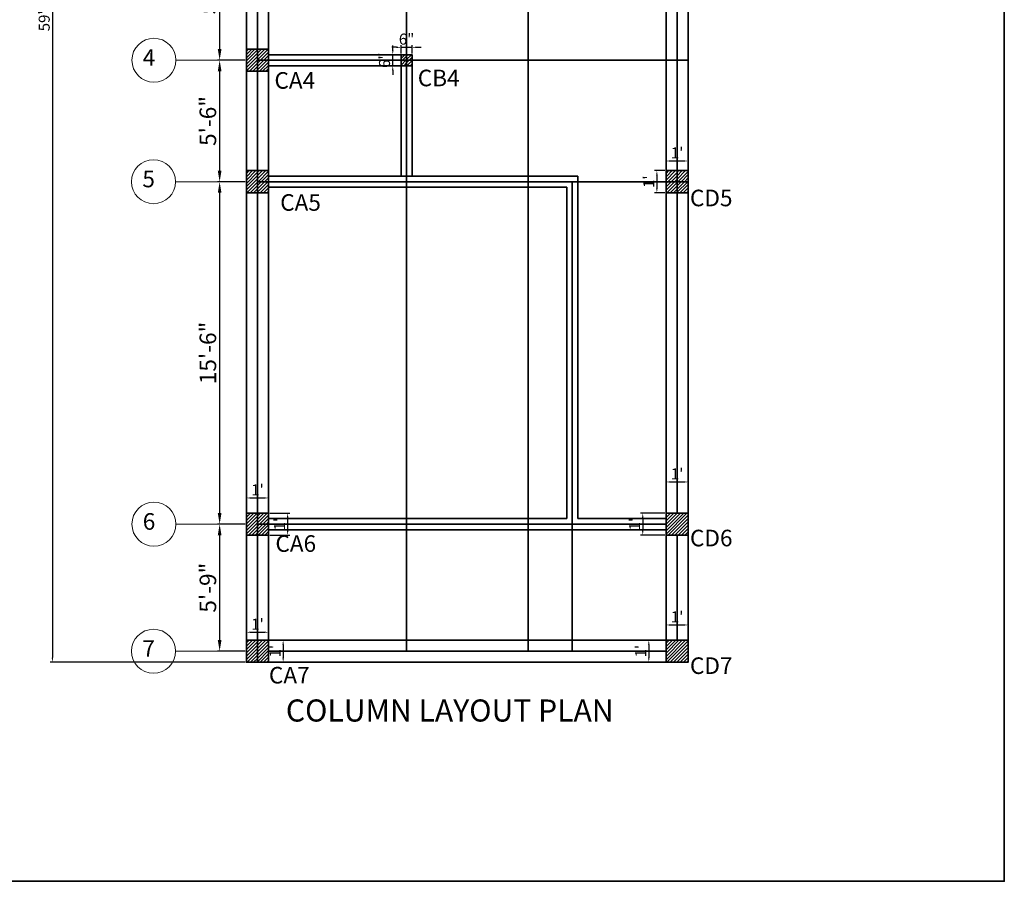
# Model space of a CAD drawing. Units: millimetres. Extents: x 20768 to 23556, y 50760 to 52704.
# Tile 34 of 36: x 23021 to 23556, y 51624 to 52092. Entities that reach past the tile are written whole.
import ezdxf

# ---------------------------------------------------------------- set-up
doc = ezdxf.new("R2010")
doc.units = ezdxf.units.MM
for name, color, linetype, lineweight in [('A-ANNO-TTLB', 7, 'Continuous', 35), ('S-ANNO-DIMS', 2, 'Continuous', 18), ('S-ANNO-TEXT', 6, 'Continuous', 18), ('S-BEAM', 3, 'Continuous', 35), ('S-COLS', 20, 'Continuous', 35), ('S-COLS-PATT', 8, 'Continuous', 13), ('S-GRID', 1, 'Continuous', 18)]:
    doc.layers.add(name, color=color, linetype=linetype, lineweight=lineweight)
doc.styles.get("Standard").update_dxf_attribs({"font": 'arial.ttf'})
doc.dimstyles.new('ISO-25', dxfattribs={"dimtxt": 6, "dimasz": 2.5, "dimexe": 1.25, "dimexo": 0.625, "dimtad": 1, "dimdec": 0, "dimlunit": 3, "dimtxsty": 'Standard', "dimcen": 2.5, "dimadec": 0, "dimazin": 0, "dimtfac": 1, "dimtdec": 0, "dimtmove": 0, "dimatfit": 3, "dimfxl": 1, "dimarcsym": 0})
pattern_1 = [(45, (1088.7427, 0), (-0.898025612, 0.898025612), [])]

# ---------------------------------------------------------------- blocks, each defined once
blk = doc.blocks.new('*D85')
at = {"layer": 'Defpoints', "color": 0, "transparency": 16777216}
for p in [(23144.01, 52129.51), (23129.44, 52069.51), (23144.01, 52069.51)]:
    blk.add_point(p, dxfattribs=at)
at = {"layer": 'S-ANNO-DIMS', "color": 0, "lineweight": -2, "transparency": 16777216}
for p, q in [((23143.39, 52129.51), (23128.19, 52129.51)), ((23129.44, 52123.51), (23129.44, 52075.51)), ((23143.39, 52069.51), (23128.19, 52069.51))]:
    blk.add_line(p, q, dxfattribs=at)
at = {"layer": 'S-ANNO-DIMS', "color": 0, "transparency": 16777216}
for points in [[(23128.44, 52123.51), (23130.44, 52123.51), (23129.44, 52129.51)], [(23128.44, 52075.51), (23130.44, 52075.51), (23129.44, 52069.51)]]:
    blk.add_solid(points, dxfattribs=at)
at = {"layer": 'S-ANNO-DIMS', "color": 0, "transparency": 16777216, "insert": (23124.24, 52099.51), "char_height": 9, "attachment_point": 5, "rotation": 90}
blk.add_mtext("5'", dxfattribs=at)
blk = doc.blocks.new('*D86')
at = {"layer": 'Defpoints', "color": 0, "transparency": 16777216}
for p in [(23144.01, 52069.51), (23129.44, 52003.51), (23144.01, 52003.51)]:
    blk.add_point(p, dxfattribs=at)
at = {"layer": 'S-ANNO-DIMS', "color": 0, "lineweight": -2, "transparency": 16777216}
for p, q in [((23143.39, 52069.51), (23128.19, 52069.51)), ((23129.44, 52063.51), (23129.44, 52009.51)), ((23143.39, 52003.51), (23128.19, 52003.51))]:
    blk.add_line(p, q, dxfattribs=at)
at = {"layer": 'S-ANNO-DIMS', "color": 0, "transparency": 16777216}
for points in [[(23128.44, 52063.51), (23130.44, 52063.51), (23129.44, 52069.51)], [(23128.44, 52009.51), (23130.44, 52009.51), (23129.44, 52003.51)]]:
    blk.add_solid(points, dxfattribs=at)
at = {"layer": 'S-ANNO-DIMS', "color": 0, "transparency": 16777216, "insert": (23124.22, 52036.51), "char_height": 9, "attachment_point": 5, "rotation": 90}
blk.add_mtext('5\'-6"', dxfattribs=at)
blk = doc.blocks.new('*D87')
at = {"layer": 'Defpoints', "color": 0, "transparency": 16777216}
for p in [(23144.01, 52003.51), (23129.44, 51817.51), (23144.01, 51817.51)]:
    blk.add_point(p, dxfattribs=at)
at = {"layer": 'S-ANNO-DIMS', "color": 0, "lineweight": -2, "transparency": 16777216}
for p, q in [((23143.39, 52003.51), (23128.19, 52003.51)), ((23129.44, 51997.51), (23129.44, 51823.51)), ((23143.39, 51817.51), (23128.19, 51817.51))]:
    blk.add_line(p, q, dxfattribs=at)
at = {"layer": 'S-ANNO-DIMS', "color": 0, "transparency": 16777216}
for points in [[(23128.44, 51997.51), (23130.44, 51997.51), (23129.44, 52003.51)], [(23128.44, 51823.51), (23130.44, 51823.51), (23129.44, 51817.51)]]:
    blk.add_solid(points, dxfattribs=at)
at = {"layer": 'S-ANNO-DIMS', "color": 0, "transparency": 16777216, "insert": (23124.22, 51910.51), "char_height": 9, "attachment_point": 5, "rotation": 90}
blk.add_mtext('15\'-6"', dxfattribs=at)
blk = doc.blocks.new('*D88')
at = {"layer": 'Defpoints', "color": 0, "transparency": 16777216}
for p in [(23144.01, 51817.51), (23129.44, 51748.51), (23144.01, 51748.51)]:
    blk.add_point(p, dxfattribs=at)
at = {"layer": 'S-ANNO-DIMS', "color": 0, "lineweight": -2, "transparency": 16777216}
for p, q in [((23143.39, 51817.51), (23128.19, 51817.51)), ((23129.44, 51811.51), (23129.44, 51754.51)), ((23143.39, 51748.51), (23128.19, 51748.51))]:
    blk.add_line(p, q, dxfattribs=at)
at = {"layer": 'S-ANNO-DIMS', "color": 0, "transparency": 16777216}
for points in [[(23128.44, 51811.51), (23130.44, 51811.51), (23129.44, 51817.51)], [(23128.44, 51754.51), (23130.44, 51754.51), (23129.44, 51748.51)]]:
    blk.add_solid(points, dxfattribs=at)
at = {"layer": 'S-ANNO-DIMS', "color": 0, "transparency": 16777216, "insert": (23124.22, 51783.01), "char_height": 9, "attachment_point": 5, "rotation": 90}
blk.add_mtext('5\'-9"', dxfattribs=at)
blk = doc.blocks.new('*D96')
at = {"layer": 'Defpoints', "color": 0, "transparency": 16777216}
for p in [(23228.01, 52072.51), (23234.01, 52076.5), (23234.01, 52072.51)]:
    blk.add_point(p, dxfattribs=at)
at = {"layer": 'S-ANNO-DIMS', "color": 0, "lineweight": -2, "transparency": 16777216}
for p, q in [((23228.01, 52073.13), (23228.01, 52077.75)), ((23234.01, 52073.13), (23234.01, 52077.75)), ((23225.51, 52076.5), (23223.01, 52076.5)), ((23228.01, 52076.5), (23234.01, 52076.5)), ((23236.51, 52076.5), (23239.01, 52076.5))]:
    blk.add_line(p, q, dxfattribs=at)
at = {"layer": 'S-ANNO-DIMS', "color": 0, "transparency": 16777216}
for points in [[(23225.51, 52076.92), (23225.51, 52076.09), (23228.01, 52076.5)], [(23236.51, 52076.92), (23236.51, 52076.09), (23234.01, 52076.5)]]:
    blk.add_solid(points, dxfattribs=at)
at = {"layer": 'S-ANNO-DIMS', "color": 0, "transparency": 16777216, "insert": (23231.01, 52080.19), "char_height": 6, "attachment_point": 5}
blk.add_mtext('6"', dxfattribs=at)
blk = doc.blocks.new('*D97')
at = {"layer": 'Defpoints', "color": 0, "transparency": 16777216}
for p in [(23223.5, 52072.51), (23228.01, 52072.51), (23228.01, 52066.51)]:
    blk.add_point(p, dxfattribs=at)
at = {"layer": 'S-ANNO-DIMS', "color": 0, "lineweight": -2, "transparency": 16777216}
for p, q in [((23227.39, 52072.51), (23222.25, 52072.51)), ((23223.5, 52075.01), (23223.5, 52077.51)), ((23223.5, 52066.51), (23223.5, 52072.51)), ((23227.39, 52066.51), (23222.25, 52066.51)), ((23223.5, 52064.01), (23223.5, 52061.51))]:
    blk.add_line(p, q, dxfattribs=at)
at = {"layer": 'S-ANNO-DIMS', "color": 0, "transparency": 16777216}
for points in [[(23223.09, 52075.01), (23223.92, 52075.01), (23223.5, 52072.51)], [(23223.09, 52064.01), (23223.92, 52064.01), (23223.5, 52066.51)]]:
    blk.add_solid(points, dxfattribs=at)
at = {"layer": 'S-ANNO-DIMS', "color": 0, "transparency": 16777216, "insert": (23219.81, 52069.51), "char_height": 6, "attachment_point": 5, "rotation": 90}
blk.add_mtext('6"', dxfattribs=at)
blk = doc.blocks.new('*D98')
at = {"layer": 'Defpoints', "color": 0, "transparency": 16777216}
for p in [(23384.01, 52014.76), (23372.01, 52009.51), (23384.01, 52009.51)]:
    blk.add_point(p, dxfattribs=at)
at = {"layer": 'S-ANNO-DIMS', "color": 0, "lineweight": -2, "transparency": 16777216}
for p, q in [((23372.01, 52010.13), (23372.01, 52016.01)), ((23374.51, 52014.76), (23381.51, 52014.76)), ((23384.01, 52010.13), (23384.01, 52016.01))]:
    blk.add_line(p, q, dxfattribs=at)
at = {"layer": 'S-ANNO-DIMS', "color": 0, "transparency": 16777216}
for points in [[(23374.51, 52015.17), (23374.51, 52014.34), (23372.01, 52014.76)], [(23381.51, 52015.17), (23381.51, 52014.34), (23384.01, 52014.76)]]:
    blk.add_solid(points, dxfattribs=at)
at = {"layer": 'S-ANNO-DIMS', "color": 0, "transparency": 16777216, "insert": (23378.01, 52018.39), "char_height": 6, "attachment_point": 5}
blk.add_mtext("1'", dxfattribs=at)
blk = doc.blocks.new('*D99')
at = {"layer": 'Defpoints', "color": 0, "transparency": 16777216}
for p in [(23372.01, 52009.51), (23367.02, 51997.51), (23372.01, 51997.51)]:
    blk.add_point(p, dxfattribs=at)
at = {"layer": 'S-ANNO-DIMS', "color": 0, "lineweight": -2, "transparency": 16777216}
for p, q in [((23371.39, 52009.51), (23365.77, 52009.51)), ((23367.02, 52007.01), (23367.02, 52000.01)), ((23371.39, 51997.51), (23365.77, 51997.51))]:
    blk.add_line(p, q, dxfattribs=at)
at = {"layer": 'S-ANNO-DIMS', "color": 0, "transparency": 16777216}
for points in [[(23366.61, 52007.01), (23367.44, 52007.01), (23367.02, 52009.51)], [(23366.61, 52000.01), (23367.44, 52000.01), (23367.02, 51997.51)]]:
    blk.add_solid(points, dxfattribs=at)
at = {"layer": 'S-ANNO-DIMS', "color": 0, "transparency": 16777216, "insert": (23363.39, 52003.51), "char_height": 6, "attachment_point": 5, "rotation": 90}
blk.add_mtext("1'", dxfattribs=at)
blk = doc.blocks.new('*D100')
at = {"layer": 'Defpoints', "color": 0, "transparency": 16777216}
for p in [(23384.01, 51762.75), (23372.01, 51754.51), (23384.01, 51754.51)]:
    blk.add_point(p, dxfattribs=at)
at = {"layer": 'S-ANNO-DIMS', "color": 0, "lineweight": -2, "transparency": 16777216}
for p, q in [((23372.01, 51755.13), (23372.01, 51764)), ((23374.51, 51762.75), (23381.51, 51762.75)), ((23384.01, 51755.13), (23384.01, 51764))]:
    blk.add_line(p, q, dxfattribs=at)
at = {"layer": 'S-ANNO-DIMS', "color": 0, "transparency": 16777216}
for points in [[(23374.51, 51763.17), (23374.51, 51762.33), (23372.01, 51762.75)], [(23381.51, 51763.17), (23381.51, 51762.33), (23384.01, 51762.75)]]:
    blk.add_solid(points, dxfattribs=at)
at = {"layer": 'S-ANNO-DIMS', "color": 0, "transparency": 16777216, "insert": (23378.01, 51766.39), "char_height": 6, "attachment_point": 5}
blk.add_mtext("1'", dxfattribs=at)
blk = doc.blocks.new('*D101')
at = {"layer": 'Defpoints', "color": 0, "transparency": 16777216}
for p in [(23372.01, 51754.51), (23362.63, 51742.51), (23372.01, 51742.51)]:
    blk.add_point(p, dxfattribs=at)
at = {"layer": 'S-ANNO-DIMS', "color": 0, "lineweight": -2, "transparency": 16777216}
for p, q in [((23371.39, 51754.51), (23361.38, 51754.51)), ((23362.63, 51752.01), (23362.63, 51745.01)), ((23371.39, 51742.51), (23361.38, 51742.51))]:
    blk.add_line(p, q, dxfattribs=at)
at = {"layer": 'S-ANNO-DIMS', "color": 0, "transparency": 16777216}
for points in [[(23362.22, 51752.01), (23363.05, 51752.01), (23362.63, 51754.51)], [(23362.22, 51745.01), (23363.05, 51745.01), (23362.63, 51742.51)]]:
    blk.add_solid(points, dxfattribs=at)
at = {"layer": 'S-ANNO-DIMS', "color": 0, "transparency": 16777216, "insert": (23359, 51748.51), "char_height": 6, "attachment_point": 5, "rotation": 90}
blk.add_mtext("1'", dxfattribs=at)
blk = doc.blocks.new('*D102')
at = {"layer": 'Defpoints', "color": 0, "transparency": 16777216}
for p in [(23156.01, 51758.8), (23144.01, 51754.51), (23156.01, 51754.51)]:
    blk.add_point(p, dxfattribs=at)
at = {"layer": 'S-ANNO-DIMS', "color": 0, "lineweight": -2, "transparency": 16777216}
for p, q in [((23144.01, 51755.13), (23144.01, 51760.05)), ((23146.51, 51758.8), (23153.51, 51758.8)), ((23156.01, 51755.13), (23156.01, 51760.05))]:
    blk.add_line(p, q, dxfattribs=at)
at = {"layer": 'S-ANNO-DIMS', "color": 0, "transparency": 16777216}
for points in [[(23146.51, 51759.21), (23146.51, 51758.38), (23144.01, 51758.8)], [(23153.51, 51759.21), (23153.51, 51758.38), (23156.01, 51758.8)]]:
    blk.add_solid(points, dxfattribs=at)
at = {"layer": 'S-ANNO-DIMS', "color": 0, "transparency": 16777216, "insert": (23150.01, 51762.43), "char_height": 6, "attachment_point": 5}
blk.add_mtext("1'", dxfattribs=at)
blk = doc.blocks.new('*D103')
at = {"layer": 'Defpoints', "color": 0, "transparency": 16777216}
for p in [(23156.01, 51754.51), (23156.01, 51742.51), (23163.95, 51742.51)]:
    blk.add_point(p, dxfattribs=at)
at = {"layer": 'S-ANNO-DIMS', "color": 0, "lineweight": -2, "transparency": 16777216}
for p, q in [((23156.64, 51754.51), (23165.2, 51754.51)), ((23163.95, 51752.01), (23163.95, 51745.01)), ((23156.64, 51742.51), (23165.2, 51742.51))]:
    blk.add_line(p, q, dxfattribs=at)
at = {"layer": 'S-ANNO-DIMS', "color": 0, "transparency": 16777216}
for points in [[(23163.53, 51752.01), (23164.37, 51752.01), (23163.95, 51754.51)], [(23163.53, 51745.01), (23164.37, 51745.01), (23163.95, 51742.51)]]:
    blk.add_solid(points, dxfattribs=at)
at = {"layer": 'S-ANNO-DIMS', "color": 0, "transparency": 16777216, "insert": (23160.31, 51748.51), "char_height": 6, "attachment_point": 5, "rotation": 90}
blk.add_mtext("1'", dxfattribs=at)
blk = doc.blocks.new('*D104')
at = {"layer": 'Defpoints', "color": 0, "transparency": 16777216}
for p in [(23156.01, 51831.73), (23144.01, 51823.51), (23156.01, 51823.51)]:
    blk.add_point(p, dxfattribs=at)
at = {"layer": 'S-ANNO-DIMS', "color": 0, "lineweight": -2, "transparency": 16777216}
for p, q in [((23144.01, 51824.13), (23144.01, 51832.98)), ((23146.51, 51831.73), (23153.51, 51831.73)), ((23156.01, 51824.13), (23156.01, 51832.98))]:
    blk.add_line(p, q, dxfattribs=at)
at = {"layer": 'S-ANNO-DIMS', "color": 0, "transparency": 16777216}
for points in [[(23146.51, 51832.14), (23146.51, 51831.31), (23144.01, 51831.73)], [(23153.51, 51832.14), (23153.51, 51831.31), (23156.01, 51831.73)]]:
    blk.add_solid(points, dxfattribs=at)
at = {"layer": 'S-ANNO-DIMS', "color": 0, "transparency": 16777216, "insert": (23150.01, 51835.36), "char_height": 6, "attachment_point": 5}
blk.add_mtext("1'", dxfattribs=at)
blk = doc.blocks.new('*D105')
at = {"layer": 'Defpoints', "color": 0, "transparency": 16777216}
for p in [(23156.01, 51823.51), (23156.01, 51811.51), (23166.38, 51811.51)]:
    blk.add_point(p, dxfattribs=at)
at = {"layer": 'S-ANNO-DIMS', "color": 0, "lineweight": -2, "transparency": 16777216}
for p, q in [((23156.64, 51823.51), (23167.63, 51823.51)), ((23166.38, 51821.01), (23166.38, 51814.01)), ((23156.64, 51811.51), (23167.63, 51811.51))]:
    blk.add_line(p, q, dxfattribs=at)
at = {"layer": 'S-ANNO-DIMS', "color": 0, "transparency": 16777216}
for points in [[(23165.96, 51821.01), (23166.8, 51821.01), (23166.38, 51823.51)], [(23165.96, 51814.01), (23166.8, 51814.01), (23166.38, 51811.51)]]:
    blk.add_solid(points, dxfattribs=at)
at = {"layer": 'S-ANNO-DIMS', "color": 0, "transparency": 16777216, "insert": (23162.74, 51817.51), "char_height": 6, "attachment_point": 5, "rotation": 90}
blk.add_mtext("1'", dxfattribs=at)
blk = doc.blocks.new('*D106')
at = {"layer": 'Defpoints', "color": 0, "transparency": 16777216}
for p in [(23384.01, 51840.43), (23372.01, 51823.51), (23384.01, 51823.51)]:
    blk.add_point(p, dxfattribs=at)
at = {"layer": 'S-ANNO-DIMS', "color": 0, "lineweight": -2, "transparency": 16777216}
for p, q in [((23372.01, 51824.13), (23372.01, 51841.68)), ((23374.51, 51840.43), (23381.51, 51840.43)), ((23384.01, 51824.13), (23384.01, 51841.68))]:
    blk.add_line(p, q, dxfattribs=at)
at = {"layer": 'S-ANNO-DIMS', "color": 0, "transparency": 16777216}
for points in [[(23374.51, 51840.84), (23374.51, 51840.01), (23372.01, 51840.43)], [(23381.51, 51840.84), (23381.51, 51840.01), (23384.01, 51840.43)]]:
    blk.add_solid(points, dxfattribs=at)
at = {"layer": 'S-ANNO-DIMS', "color": 0, "transparency": 16777216, "insert": (23378.01, 51844.06), "char_height": 6, "attachment_point": 5}
blk.add_mtext("1'", dxfattribs=at)
blk = doc.blocks.new('*D107')
at = {"layer": 'Defpoints', "color": 0, "transparency": 16777216}
for p in [(23372.01, 51823.51), (23359.35, 51811.51), (23372.01, 51811.51)]:
    blk.add_point(p, dxfattribs=at)
at = {"layer": 'S-ANNO-DIMS', "color": 0, "lineweight": -2, "transparency": 16777216}
for p, q in [((23371.39, 51823.51), (23358.1, 51823.51)), ((23359.35, 51821.01), (23359.35, 51814.01)), ((23371.39, 51811.51), (23358.1, 51811.51))]:
    blk.add_line(p, q, dxfattribs=at)
at = {"layer": 'S-ANNO-DIMS', "color": 0, "transparency": 16777216}
for points in [[(23358.93, 51821.01), (23359.77, 51821.01), (23359.35, 51823.51)], [(23358.93, 51814.01), (23359.77, 51814.01), (23359.35, 51811.51)]]:
    blk.add_solid(points, dxfattribs=at)
at = {"layer": 'S-ANNO-DIMS', "color": 0, "transparency": 16777216, "insert": (23355.71, 51817.51), "char_height": 6, "attachment_point": 5, "rotation": 90}
blk.add_mtext("1'", dxfattribs=at)
blk = doc.blocks.new('GRID-BUBBLE')
blk.add_line((47.87, 11.93), (23.87, 11.93))
blk.add_circle((11.93, 11.93), 11.93)
blk = doc.blocks.new('*D228')
at = {"layer": 'Defpoints', "color": 0, "transparency": 16777216}
for p in [(23144.01, 52450.51), (23038.57, 51742.51), (23144.01, 51742.51)]:
    blk.add_point(p, dxfattribs=at)
at = {"layer": 'S-ANNO-DIMS', "color": 0, "lineweight": -2, "transparency": 16777216}
for p, q in [((23143.39, 52450.51), (23037.32, 52450.51)), ((23038.57, 52448.01), (23038.57, 51745.01)), ((23143.39, 51742.51), (23037.32, 51742.51))]:
    blk.add_line(p, q, dxfattribs=at)
at = {"layer": 'S-ANNO-DIMS', "color": 0, "transparency": 16777216}
for points in [[(23038.16, 52448.01), (23038.99, 52448.01), (23038.57, 52450.51)], [(23038.16, 51745.01), (23038.99, 51745.01), (23038.57, 51742.51)]]:
    blk.add_solid(points, dxfattribs=at)
at = {"layer": 'S-ANNO-DIMS', "color": 0, "transparency": 16777216, "insert": (23034.88, 52096.51), "char_height": 6, "attachment_point": 5, "rotation": 90}
blk.add_mtext('59\'-0"', dxfattribs=at)

msp = doc.modelspace()

# ---------------------------------------------------------------- hatches: boundary and pattern name
at = {"layer": 'S-COLS-PATT'}
h = msp.add_hatch(dxfattribs=at)
h.set_pattern_fill('ANSI31', color=256, scale=0.4)
h.set_pattern_definition(pattern_1)
h.paths.add_polyline_path([(23150.01, 52075.51), (23144.01, 52075.51), (23144.01, 52063.51), (23150.01, 52063.51)])
h = msp.add_hatch(dxfattribs=at)
h.set_pattern_fill('ANSI31', color=256, scale=0.4)
h.set_pattern_definition(pattern_1)
h.paths.add_polyline_path([(23156.01, 52075.51), (23150.01, 52075.51), (23150.01, 52069.51), (23156.01, 52069.51)])
h = msp.add_hatch(dxfattribs=at)
h.set_pattern_fill('ANSI31', color=256, scale=0.4)
h.set_pattern_definition(pattern_1)
h.paths.add_polyline_path([(23231.01, 52072.51), (23228.01, 52072.51), (23228.01, 52069.51), (23231.01, 52069.51)])
h = msp.add_hatch(dxfattribs=at)
h.set_pattern_fill('ANSI31', color=256, scale=0.4)
h.set_pattern_definition(pattern_1)
h.paths.add_polyline_path([(23234.01, 52072.51), (23231.01, 52072.51), (23231.01, 52069.51), (23234.01, 52069.51)], flags=17)
h = msp.add_hatch(dxfattribs=at)
h.set_pattern_fill('ANSI31', color=256, scale=0.4)
h.set_pattern_definition(pattern_1)
h.paths.add_polyline_path([(23156.01, 52069.51), (23150.01, 52069.51), (23150.01, 52063.51), (23156.01, 52063.51)])
h = msp.add_hatch(dxfattribs=at)
h.set_pattern_fill('ANSI31', color=256, scale=0.4)
h.set_pattern_definition(pattern_1)
h.paths.add_polyline_path([(23231.01, 52069.51), (23228.01, 52069.51), (23228.01, 52066.51), (23231.01, 52066.51)])
h = msp.add_hatch(dxfattribs=at)
h.set_pattern_fill('ANSI31', color=256, scale=0.4)
h.set_pattern_definition(pattern_1)
h.paths.add_polyline_path([(23234.01, 52069.51), (23231.01, 52069.51), (23231.01, 52066.51), (23234.01, 52066.51)])
h = msp.add_hatch(dxfattribs=at)
h.set_pattern_fill('ANSI31', color=256, scale=0.4)
h.set_pattern_definition(pattern_1)
h.paths.add_polyline_path([(23150.01, 52009.51), (23144.01, 52009.51), (23144.01, 51997.51), (23150.01, 51997.51)])
h = msp.add_hatch(dxfattribs=at)
h.set_pattern_fill('ANSI31', color=256, scale=0.4)
h.set_pattern_definition(pattern_1)
h.paths.add_polyline_path([(23156.01, 52009.51), (23150.01, 52009.51), (23150.01, 52003.51), (23156.01, 52003.51)])
h = msp.add_hatch(dxfattribs=at)
h.set_pattern_fill('ANSI31', color=256, scale=0.4)
h.set_pattern_definition(pattern_1)
h.paths.add_polyline_path([(23378.01, 52009.51), (23372.01, 52009.51), (23372.01, 52003.51), (23378.01, 52003.51)])
h = msp.add_hatch(dxfattribs=at)
h.set_pattern_fill('ANSI31', color=256, scale=0.4)
h.set_pattern_definition(pattern_1)
h.paths.add_polyline_path([(23384.01, 52009.51), (23378.01, 52009.51), (23378.01, 52003.51), (23384.01, 52003.51)])
h = msp.add_hatch(dxfattribs=at)
h.set_pattern_fill('ANSI31', color=256, scale=0.4)
h.set_pattern_definition(pattern_1)
h.paths.add_polyline_path([(23156.01, 52003.51), (23150.01, 52003.51), (23150.01, 51997.51), (23156.01, 51997.51)])
h = msp.add_hatch(dxfattribs=at)
h.set_pattern_fill('ANSI31', color=256, scale=0.4)
h.set_pattern_definition(pattern_1)
h.paths.add_polyline_path([(23378.01, 52003.51), (23372.01, 52003.51), (23372.01, 51997.51), (23378.01, 51997.51)])
h = msp.add_hatch(dxfattribs=at)
h.set_pattern_fill('ANSI31', color=256, scale=0.4)
h.set_pattern_definition(pattern_1)
h.paths.add_polyline_path([(23384.01, 52003.51), (23378.01, 52003.51), (23378.01, 51997.51), (23384.01, 51997.51)])
h = msp.add_hatch(dxfattribs=at)
h.set_pattern_fill('ANSI31', color=256, scale=0.4)
h.set_pattern_definition(pattern_1)
h.paths.add_polyline_path([(23150.01, 51823.51), (23144.01, 51823.51), (23144.01, 51811.51), (23150.01, 51811.51)])
h = msp.add_hatch(dxfattribs=at)
h.set_pattern_fill('ANSI31', color=256, scale=0.4)
h.set_pattern_definition(pattern_1)
h.paths.add_polyline_path([(23156.01, 51823.51), (23150.01, 51823.51), (23150.01, 51817.51), (23156.01, 51817.51)])
h = msp.add_hatch(dxfattribs=at)
h.set_pattern_fill('ANSI31', color=256, scale=0.4)
h.set_pattern_definition(pattern_1)
h.paths.add_polyline_path([(23384.01, 51823.51), (23372.01, 51823.51), (23372.01, 51811.51), (23384.01, 51811.51)])
h = msp.add_hatch(dxfattribs=at)
h.set_pattern_fill('ANSI31', color=256, scale=0.4)
h.set_pattern_definition(pattern_1)
h.paths.add_polyline_path([(23156.01, 51817.51), (23150.01, 51817.51), (23150.01, 51811.51), (23156.01, 51811.51)])
h = msp.add_hatch(dxfattribs=at)
h.set_pattern_fill('ANSI31', color=256, scale=0.4)
h.set_pattern_definition(pattern_1)
h.paths.add_polyline_path([(23150.01, 51754.51), (23144.01, 51754.51), (23144.01, 51742.51), (23150.01, 51742.51)])
h = msp.add_hatch(dxfattribs=at)
h.set_pattern_fill('ANSI31', color=256, scale=0.4)
h.set_pattern_definition(pattern_1)
h.paths.add_polyline_path([(23156.01, 51754.51), (23150.01, 51754.51), (23150.01, 51742.51), (23156.01, 51742.51)])
h = msp.add_hatch(dxfattribs=at)
h.set_pattern_fill('ANSI31', color=256, scale=0.4)
h.set_pattern_definition(pattern_1)
h.paths.add_polyline_path([(23384.01, 51754.51), (23372.01, 51754.51), (23372.01, 51742.51), (23384.01, 51742.51)])

# ---------------------------------------------------------------- linework, layer by layer
at = {"layer": 'A-ANNO-TTLB'}
msp.add_lwpolyline([(20768.14, 52703.98), (23555.8, 52703.98), (23555.8, 51623.53), (20768.14, 51623.53)], close=True, dxfattribs=at)
at = {"layer": 'S-BEAM'}
for p, q in [((23144.01, 52450.51), (23144.01, 51742.51)), ((23156.01, 52450.51), (23156.01, 51742.51)), ((23231.01, 52450.51), (23231.01, 51748.51)), ((23297.01, 52450.51), (23297.01, 51748.51)), ((23372.01, 52450.51), (23372.01, 51742.51)), ((23384.01, 52450.51), (23384.01, 51742.51)), ((23150.01, 52444.51), (23150.01, 51742.51)), ((23378.01, 52123.51), (23378.01, 51823.51)), ((23156.01, 52072.51), (23234.01, 52072.51)), ((23228.01, 52072.51), (23228.01, 52006.51)), ((23234.01, 52072.51), (23234.01, 52006.51)), ((23150.01, 52069.51), (23384.01, 52069.51)), ((23156.01, 52066.51), (23234.01, 52066.51)), ((23150.01, 52003.51), (23384.01, 52003.51)), ((23156.01, 52006.51), (23324.01, 52006.51)), ((23321.01, 52003.51), (23321.01, 51748.51)), ((23324.01, 52006.51), (23324.01, 51820.51)), ((23156.01, 52000.51), (23318.01, 52000.51)), ((23318.01, 52000.51), (23318.01, 51820.51)), ((23150.01, 51817.51), (23372.01, 51817.51)), ((23156.01, 51820.51), (23318.01, 51820.51)), ((23324.01, 51820.51), (23372.01, 51820.51)), ((23156.01, 51814.51), (23372.01, 51814.51)), ((23378.01, 51811.51), (23378.01, 51754.51)), ((23156.01, 51754.51), (23384.01, 51754.51)), ((23156.01, 51748.51), (23372.01, 51748.51)), ((23144.01, 51742.51), (23384.01, 51742.51))]:
    msp.add_line(p, q, dxfattribs=at)
at = {"layer": 'S-COLS'}
for points in [[(23156.01, 52075.51), (23144.01, 52075.51), (23144.01, 52063.51), (23156.01, 52063.51)], [(23228.01, 52072.51), (23234.01, 52072.51), (23234.01, 52066.51), (23228.01, 52066.51)], [(23156.01, 52009.51), (23144.01, 52009.51), (23144.01, 51997.51), (23156.01, 51997.51)], [(23372.01, 52009.51), (23384.01, 52009.51), (23384.01, 51997.51), (23372.01, 51997.51)], [(23156.01, 51823.51), (23144.01, 51823.51), (23144.01, 51811.51), (23156.01, 51811.51)], [(23372.01, 51823.51), (23384.01, 51823.51), (23384.01, 51811.51), (23372.01, 51811.51)], [(23156.01, 51754.51), (23144.01, 51754.51), (23144.01, 51742.51), (23156.01, 51742.51)], [(23372.01, 51754.51), (23384.01, 51754.51), (23384.01, 51742.51), (23372.01, 51742.51)]]:
    msp.add_lwpolyline(points, close=True, dxfattribs=at)

# ---------------------------------------------------------------- block references
at = {"layer": 'S-GRID'}
for p in [(23081.78, 52057.57), (23081.57, 51991.57), (23081.78, 51805.57), (23081.57, 51736.57)]:
    msp.add_blockref('GRID-BUBBLE', p, dxfattribs=at)

# ---------------------------------------------------------------- texts
at = {"layer": 'S-ANNO-TEXT', "attachment_point": 1}
for s, width, insert, char_height in [('  4', 27.5349, (23082.17, 52075.48), 9), ('CA4', 15.3341, (23159.22, 52063.02), 9), ('CB4', 15.3341, (23237.1, 52064.35), 9), ('  5', 27.5349, (23081.96, 52009.48), 9), ('CD5', 15.3341, (23385.01, 51999.17), 9), ('CA5', 15.3341, (23162.34, 51996.73), 9), ('  6', 27.5349, (23082.17, 51823.48), 9), ('CA6', 15.3341, (23159.75, 51811.48), 9), ('CD6', 15.3341, (23385.01, 51814.47), 9), ('  7', 27.5349, (23081.96, 51754.48), 9), ('CD7', 15.3341, (23385.01, 51745.15), 9), ('CA7', 15.3341, (23156.23, 51739.98), 9), ('COLUMN LAYOUT PLAN', 241.5904, (23165.42, 51722.3), 12)]:
    msp.add_mtext_dynamic_manual_height_columns(s, width=width, gutter_width=12.5, heights=[0], dxfattribs=dict(at, insert=insert, char_height=char_height))

# ---------------------------------------------------------------- dimensions: what is measured, and where the dimension line sits
at = {"layer": 'S-ANNO-DIMS'}
for base, p1, p2, override, picture, middle in [((23038.57, 51742.51), (23144.01, 52450.51), (23144.01, 51742.51), {"dimdec": 1, "dimlfac": 1, "dimrnd": 0, "dimzin": 1, "dimdsep": 46, "dimlunit": 4, "dimfrac": 2}, '*D228', (23034.88, 52096.51)), ((23129.44, 52069.51), (23144.01, 52129.51), (23144.01, 52069.51), {"dimtxt": 9, "dimasz": 6, "dimclrd": 0, "dimclre": 0, "dimclrt": 0}, '*D85', (23124.24, 52099.51)), ((23129.44, 52003.51), (23144.01, 52069.51), (23144.01, 52003.51), {"dimtxt": 9, "dimasz": 6, "dimclrd": 0, "dimclre": 0, "dimclrt": 0}, '*D86', (23124.22, 52036.51)), ((23367.02, 51997.51), (23372.01, 52009.51), (23372.01, 51997.51), {"dimclrd": 0, "dimclre": 0, "dimclrt": 0}, '*D99', (23363.39, 52003.51)), ((23129.44, 51817.51), (23144.01, 52003.51), (23144.01, 51817.51), {"dimtxt": 9, "dimasz": 6, "dimclrd": 0, "dimclre": 0, "dimclrt": 0}, '*D87', (23124.22, 51910.51)), ((23166.38, 51811.51), (23156.01, 51823.51), (23156.01, 51811.51), {"dimclrd": 0, "dimclre": 0, "dimclrt": 0}, '*D105', (23162.74, 51817.51)), ((23359.35, 51811.51), (23372.01, 51823.51), (23372.01, 51811.51), {"dimclrd": 0, "dimclre": 0, "dimclrt": 0}, '*D107', (23355.71, 51817.51)), ((23129.44, 51748.51), (23144.01, 51817.51), (23144.01, 51748.51), {"dimtxt": 9, "dimasz": 6, "dimclrd": 0, "dimclre": 0, "dimclrt": 0}, '*D88', (23124.22, 51783.01)), ((23163.95, 51742.51), (23156.01, 51754.51), (23156.01, 51742.51), {"dimclrd": 0, "dimclre": 0, "dimclrt": 0}, '*D103', (23160.31, 51748.51)), ((23362.63, 51742.51), (23372.01, 51754.51), (23372.01, 51742.51), {"dimclrd": 0, "dimclre": 0, "dimclrt": 0}, '*D101', (23359, 51748.51))]:
    dim = msp.add_linear_dim(base=base, p1=p1, p2=p2, angle=90, dimstyle='ISO-25', override=override, dxfattribs=at)
    dim.commit()
    dim.dimension.update_dxf_attribs({"geometry": picture, "text_midpoint": middle})
dim = msp.add_linear_dim(base=(23234.01, 52076.5), p1=(23228.01, 52072.51), p2=(23234.01, 52072.51), dimstyle='ISO-25', override={"dimclrd": 0, "dimclre": 0, "dimclrt": 0}, dxfattribs=at)
dim.commit()
dim.dimension.update_dxf_attribs({"geometry": '*D96', "text_midpoint": (23231.01, 52076.5), "dimtype": 160})
dim = msp.add_linear_dim(base=(23223.5, 52072.51), p1=(23228.01, 52066.51), p2=(23228.01, 52072.51), angle=90, dimstyle='ISO-25', override={"dimclrd": 0, "dimclre": 0, "dimclrt": 0}, dxfattribs=at)
dim.commit()
dim.dimension.update_dxf_attribs({"geometry": '*D97', "text_midpoint": (23223.5, 52069.51), "dimtype": 160})
for base, p1, p2, picture, middle in [((23384.01, 52014.76), (23372.01, 52009.51), (23384.01, 52009.51), '*D98', (23378.01, 52018.39)), ((23384.01, 51840.43), (23372.01, 51823.51), (23384.01, 51823.51), '*D106', (23378.01, 51844.06)), ((23156.01, 51831.73), (23144.01, 51823.51), (23156.01, 51823.51), '*D104', (23150.01, 51835.36)), ((23384.01, 51762.75), (23372.01, 51754.51), (23384.01, 51754.51), '*D100', (23378.01, 51766.39)), ((23156.01, 51758.8), (23144.01, 51754.51), (23156.01, 51754.51), '*D102', (23150.01, 51762.43))]:
    dim = msp.add_linear_dim(base=base, p1=p1, p2=p2, dimstyle='ISO-25', override={"dimclrd": 0, "dimclre": 0, "dimclrt": 0}, dxfattribs=at)
    dim.commit()
    dim.dimension.update_dxf_attribs({"geometry": picture, "text_midpoint": middle})

doc.saveas('drawing.dxf')
